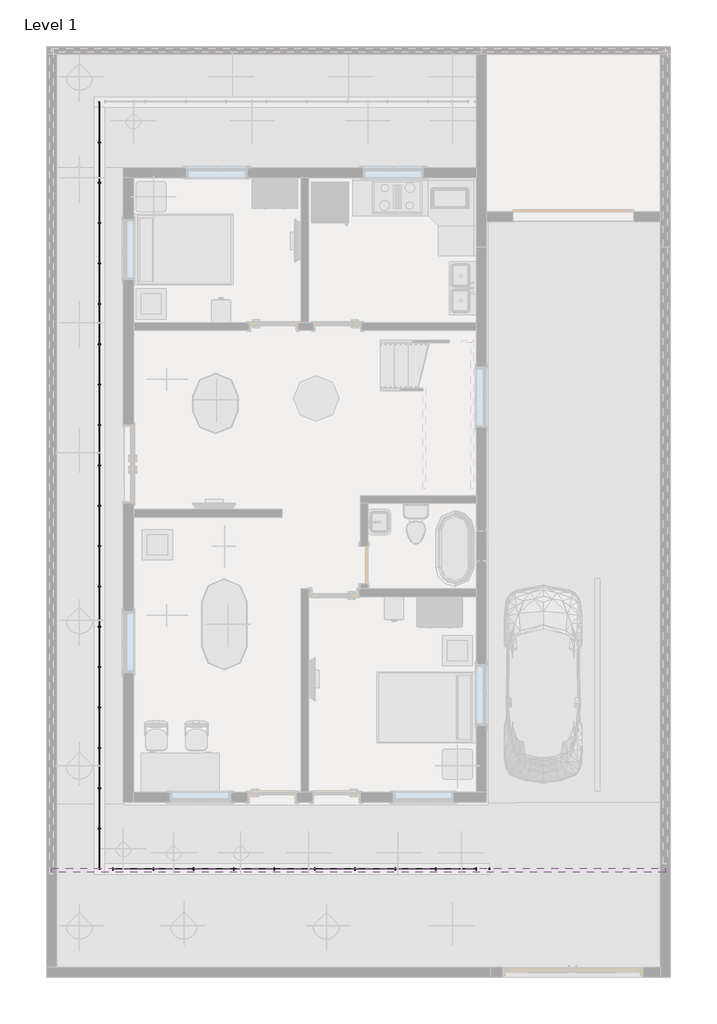
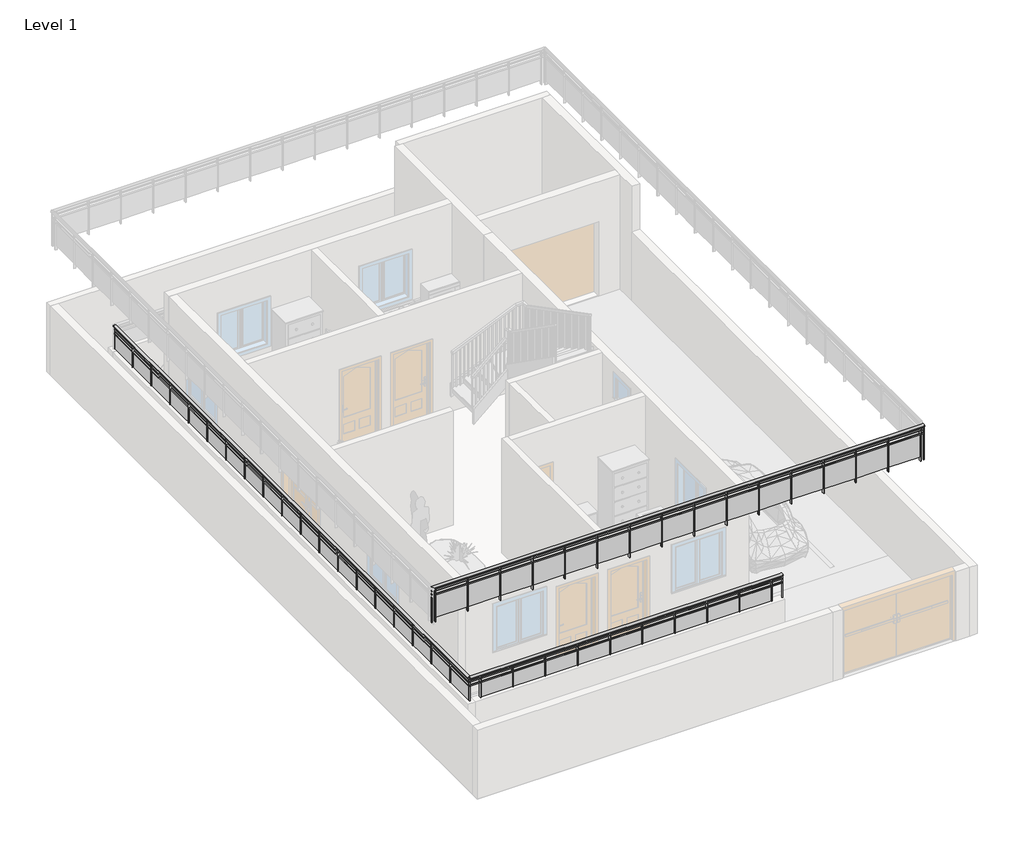
# One storey, part 2 of 5: 3 railings.
"""IFC4 building model written with IfcOpenShell, lengths in millimetres."""

from ifc_helpers import new_model, si_unit, point, frame, origin, place, context, project, spatial, polyline, ellipse_curve, trimmed, outline, extrude, element, save
from ifc_brep_helpers import plane_surface, extruded_surface, advanced_brep

model = new_model("IFC4")

# Units and contexts
model_context = context("Model", 3, world=origin())
ifc_project = project(units=[si_unit("LENGTHUNIT", "METRE", prefix="MILLI")], contexts=[model_context])

# Site, building, storey
site = spatial("IfcSite", under=ifc_project)
building = spatial("IfcBuilding", under=site)
storey = spatial("IfcBuildingStorey", under=building, Name="Level 1", Elevation=0.0)

# Railings
placement = place(None, origin())
element("IfcRailing", 1, ObjectType="Glass Panel - Bottom Fill", at=placement, inside=storey, context=model_context, shape_type="SolidModel", body=[
    advanced_brep(
    [(-10070.9350785, -4835.5966995, 1524.0), (-10070.9350785, -4911.7966995, 1524.0), (-2209.6350785, -4835.5966995, 1524.0), (-2209.6350785, -4911.7966995, 1524.0)],
    [
        (0, 1, ellipse_curve(frame((-10070.9350785, -4873.6966995, 1524.0), z_axis=(-1.0, 0.0, 0.0), x_axis=(0.0, -1.0, 0.0)), 38.1, 28.575)),
        (1, 0, ellipse_curve(frame((-10070.9350785, -4873.6966995, 1524.0), z_axis=(-1.0, 0.0, 0.0), x_axis=(0.0, -1.0, 0.0)), 38.1, 28.575)),
        (2, 3, ellipse_curve(frame((-2209.6350785, -4873.6966995, 1524.0), z_axis=(1.0, 0.0, 0.0), x_axis=(0.0, -1.0, 0.0)), 38.1, 28.575)),
        (3, 2, ellipse_curve(frame((-2209.6350785, -4873.6966995, 1524.0), z_axis=(1.0, 0.0, 0.0), x_axis=(0.0, -1.0, 0.0)), 38.1, 28.575)),
        (0, 2),
        (3, 1),
    ],
    [
        plane_surface(frame((-10070.9350785, -4873.6966995, 1524.0), z_axis=(-1.0, 0.0, 0.0), x_axis=(0.0, 1.0, 0.0))),
        plane_surface(frame((-2209.6350785, -4873.6966995, 1524.0), z_axis=(1.0, 0.0, 0.0), x_axis=(0.0, 1.0, 0.0))),
        extruded_surface(trimmed(ellipse_curve(frame((-2209.6350785, -4873.6966995, 1524.0), z_axis=(-1.0, 0.0, 0.0), x_axis=(0.0, -1.0, 0.0)), 38.1, 28.575), [point((-2209.6350785, -4835.5966995, 1524.0))], [point((-2209.6350785, -4911.7966995, 1524.0))], True, "CARTESIAN"), (-7861.300000000001, 0.0, 0.0), 7861.300000000001),
        extruded_surface(trimmed(ellipse_curve(frame((-2209.6350785, -4873.6966995, 1524.0), z_axis=(-1.0, 0.0, 0.0), x_axis=(0.0, -1.0, 0.0)), 38.1, 28.575), [point((-2209.6350785, -4911.7966995, 1524.0))], [point((-2209.6350785, -4835.5966995, 1524.0))], True, "CARTESIAN"), (-7861.300000000001, 0.0, 0.0), 7861.300000000001),
    ],
    [
        (0, [[1, 2]]),
        (1, [[3, 4]]),
        (2, [[-1, 5, -4, 6]]),
        (3, [[-2, -6, -3, -5]]),
    ],
),
    extrude(outline(polyline([(-10070.9350785, -4886.3966995), (-10070.9350785, -4860.9966995), (-2209.6350785, -4860.9966995), (-2209.6350785, -4886.3966995), (-10070.9350785, -4886.3966995)])), frame((0.0, 0.0, 1409.7), z_axis=(0.0, 0.0, 1.0), x_axis=(1.0, 0.0, 0.0)), (0.0, 0.0, 1.0), 25.4),
    extrude(outline(polyline([(-10070.9350785, -4886.3966995), (-10070.9350785, -4860.9966995), (-2209.6350785, -4860.9966995), (-2209.6350785, -4886.3966995), (-10070.9350785, -4886.3966995)])), frame((0.0, 0.0, 1308.1), z_axis=(0.0, 0.0, 1.0), x_axis=(1.0, 0.0, 0.0)), (0.0, 0.0, 1.0), 25.4),
    extrude(outline(polyline([(-2489.0350785, -4899.0966995), (-2489.0350785, -4848.2966995), (-2476.3350785, -4848.2966995), (-2476.3350785, -4899.0966995), (-2489.0350785, -4899.0966995)])), frame((0.0, 0.0, 609.6), z_axis=(0.0, 0.0, 1.0), x_axis=(1.0, 0.0, 0.0)), (0.0, 0.0, 1.0), 885.6788223),
    extrude(outline(polyline([(-3295.4850785, -4867.1615425), (-2482.6850785, -4867.1615425), (-2482.6850785, -4873.5115425), (-3295.4850785, -4873.5115425), (-3295.4850785, -4867.1615425)])), frame((0.0, 0.0, 711.2), z_axis=(0.0, 0.0, 1.0), x_axis=(1.0, 0.0, 0.0)), (0.0, 0.0, 1.0), 596.9),
    extrude(outline(polyline([(-3301.8350785, -4899.0966995), (-3301.8350785, -4848.2966995), (-3289.1350785, -4848.2966995), (-3289.1350785, -4899.0966995), (-3301.8350785, -4899.0966995)])), frame((0.0, 0.0, 609.6), z_axis=(0.0, 0.0, 1.0), x_axis=(1.0, 0.0, 0.0)), (0.0, 0.0, 1.0), 885.6788223),
    extrude(outline(polyline([(-4108.2850785, -4867.1615425), (-3295.4850785, -4867.1615425), (-3295.4850785, -4873.5115425), (-4108.2850785, -4873.5115425), (-4108.2850785, -4867.1615425)])), frame((0.0, 0.0, 711.2), z_axis=(0.0, 0.0, 1.0), x_axis=(1.0, 0.0, 0.0)), (0.0, 0.0, 1.0), 596.9),
    extrude(outline(polyline([(-4114.6350785, -4899.0966995), (-4114.6350785, -4848.2966995), (-4101.9350785, -4848.2966995), (-4101.9350785, -4899.0966995), (-4114.6350785, -4899.0966995)])), frame((0.0, 0.0, 609.6), z_axis=(0.0, 0.0, 1.0), x_axis=(1.0, 0.0, 0.0)), (0.0, 0.0, 1.0), 885.6788223),
    extrude(outline(polyline([(-4921.0850785, -4867.1615425), (-4108.2850785, -4867.1615425), (-4108.2850785, -4873.5115425), (-4921.0850785, -4873.5115425), (-4921.0850785, -4867.1615425)])), frame((0.0, 0.0, 711.2), z_axis=(0.0, 0.0, 1.0), x_axis=(1.0, 0.0, 0.0)), (0.0, 0.0, 1.0), 596.9),
    extrude(outline(polyline([(-4927.4350785, -4899.0966995), (-4927.4350785, -4848.2966995), (-4914.7350785, -4848.2966995), (-4914.7350785, -4899.0966995), (-4927.4350785, -4899.0966995)])), frame((0.0, 0.0, 609.6), z_axis=(0.0, 0.0, 1.0), x_axis=(1.0, 0.0, 0.0)), (0.0, 0.0, 1.0), 885.6788223),
    extrude(outline(polyline([(-5733.8850785, -4867.1615425), (-4921.0850785, -4867.1615425), (-4921.0850785, -4873.5115425), (-5733.8850785, -4873.5115425), (-5733.8850785, -4867.1615425)])), frame((0.0, 0.0, 711.2), z_axis=(0.0, 0.0, 1.0), x_axis=(1.0, 0.0, 0.0)), (0.0, 0.0, 1.0), 596.9),
    extrude(outline(polyline([(-5740.2350785, -4899.0966995), (-5740.2350785, -4848.2966995), (-5727.5350785, -4848.2966995), (-5727.5350785, -4899.0966995), (-5740.2350785, -4899.0966995)])), frame((0.0, 0.0, 609.6), z_axis=(0.0, 0.0, 1.0), x_axis=(1.0, 0.0, 0.0)), (0.0, 0.0, 1.0), 885.6788223),
    extrude(outline(polyline([(-6546.6850785, -4867.1615425), (-5733.8850785, -4867.1615425), (-5733.8850785, -4873.5115425), (-6546.6850785, -4873.5115425), (-6546.6850785, -4867.1615425)])), frame((0.0, 0.0, 711.2), z_axis=(0.0, 0.0, 1.0), x_axis=(1.0, 0.0, 0.0)), (0.0, 0.0, 1.0), 596.9),
    extrude(outline(polyline([(-6553.0350785, -4899.0966995), (-6553.0350785, -4848.2966995), (-6540.3350785, -4848.2966995), (-6540.3350785, -4899.0966995), (-6553.0350785, -4899.0966995)])), frame((0.0, 0.0, 609.6), z_axis=(0.0, 0.0, 1.0), x_axis=(1.0, 0.0, 0.0)), (0.0, 0.0, 1.0), 885.6788223),
    extrude(outline(polyline([(-7359.4850785, -4867.1615425), (-6546.6850785, -4867.1615425), (-6546.6850785, -4873.5115425), (-7359.4850785, -4873.5115425), (-7359.4850785, -4867.1615425)])), frame((0.0, 0.0, 711.2), z_axis=(0.0, 0.0, 1.0), x_axis=(1.0, 0.0, 0.0)), (0.0, 0.0, 1.0), 596.9),
    extrude(outline(polyline([(-7365.8350785, -4899.0966995), (-7365.8350785, -4848.2966995), (-7353.1350785, -4848.2966995), (-7353.1350785, -4899.0966995), (-7365.8350785, -4899.0966995)])), frame((0.0, 0.0, 609.6), z_axis=(0.0, 0.0, 1.0), x_axis=(1.0, 0.0, 0.0)), (0.0, 0.0, 1.0), 885.6788223),
    extrude(outline(polyline([(-8172.2850785, -4867.1615425), (-7359.4850785, -4867.1615425), (-7359.4850785, -4873.5115425), (-8172.2850785, -4873.5115425), (-8172.2850785, -4867.1615425)])), frame((0.0, 0.0, 711.2), z_axis=(0.0, 0.0, 1.0), x_axis=(1.0, 0.0, 0.0)), (0.0, 0.0, 1.0), 596.9),
    extrude(outline(polyline([(-8178.6350785, -4899.0966995), (-8178.6350785, -4848.2966995), (-8165.9350785, -4848.2966995), (-8165.9350785, -4899.0966995), (-8178.6350785, -4899.0966995)])), frame((0.0, 0.0, 609.6), z_axis=(0.0, 0.0, 1.0), x_axis=(1.0, 0.0, 0.0)), (0.0, 0.0, 1.0), 885.6788223),
    extrude(outline(polyline([(-8985.0850785, -4867.1615425), (-8172.2850785, -4867.1615425), (-8172.2850785, -4873.5115425), (-8985.0850785, -4873.5115425), (-8985.0850785, -4867.1615425)])), frame((0.0, 0.0, 711.2), z_axis=(0.0, 0.0, 1.0), x_axis=(1.0, 0.0, 0.0)), (0.0, 0.0, 1.0), 596.9),
    extrude(outline(polyline([(-8991.4350785, -4899.0966995), (-8991.4350785, -4848.2966995), (-8978.7350785, -4848.2966995), (-8978.7350785, -4899.0966995), (-8991.4350785, -4899.0966995)])), frame((0.0, 0.0, 609.6), z_axis=(0.0, 0.0, 1.0), x_axis=(1.0, 0.0, 0.0)), (0.0, 0.0, 1.0), 885.6788223),
    extrude(outline(polyline([(-9797.8850785, -4867.1615425), (-8985.0850785, -4867.1615425), (-8985.0850785, -4873.5115425), (-9797.8850785, -4873.5115425), (-9797.8850785, -4867.1615425)])), frame((0.0, 0.0, 711.2), z_axis=(0.0, 0.0, 1.0), x_axis=(1.0, 0.0, 0.0)), (0.0, 0.0, 1.0), 596.9),
    extrude(outline(polyline([(-9804.2350785, -4899.0966995), (-9804.2350785, -4848.2966995), (-9791.5350785, -4848.2966995), (-9791.5350785, -4899.0966995), (-9804.2350785, -4899.0966995)])), frame((0.0, 0.0, 609.6), z_axis=(0.0, 0.0, 1.0), x_axis=(1.0, 0.0, 0.0)), (0.0, 0.0, 1.0), 885.6788223),
    extrude(outline(polyline([(-2222.3350785, -4883.2216995), (-2222.3350785, -4864.1716995), (-2203.2850785, -4864.1716995), (-2203.2850785, -4883.2216995), (-2222.3350785, -4883.2216995)])), frame((0.0, 0.0, 609.6), z_axis=(0.0, 0.0, 1.0), x_axis=(1.0, 0.0, 0.0)), (0.0, 0.0, 1.0), 885.6788223),
    extrude(outline(polyline([(-10077.2850785, -4883.2216995), (-10077.2850785, -4864.1716995), (-10058.2350785, -4864.1716995), (-10058.2350785, -4883.2216995), (-10077.2850785, -4883.2216995)])), frame((0.0, 0.0, 609.6), z_axis=(0.0, 0.0, 1.0), x_axis=(1.0, 0.0, 0.0)), (0.0, 0.0, 1.0), 885.6788223),
])
element("IfcRailing", 2, ObjectType="Glass Panel - Bottom Fill", at=placement, inside=storey, context=model_context, shape_type="SolidModel", body=[
    advanced_brep(
    [(-10109.0350785, -4873.6966995, 1524.0), (-10032.8350785, -4873.6966995, 1524.0), (-10109.0350785, 10569.5033005, 1524.0), (-10032.8350785, 10569.5033005, 1524.0)],
    [
        (0, 1, ellipse_curve(frame((-10070.9350785, -4873.6966995, 1524.0), z_axis=(0.0, -1.0, 0.0), x_axis=(1.0, 0.0, 0.0)), 38.1, 28.575)),
        (1, 0, ellipse_curve(frame((-10070.9350785, -4873.6966995, 1524.0), z_axis=(0.0, -1.0, 0.0), x_axis=(1.0, 0.0, 0.0)), 38.1, 28.575)),
        (2, 3, ellipse_curve(frame((-10070.9350785, 10569.5033005, 1524.0), z_axis=(0.0, 1.0, 0.0), x_axis=(1.0, 0.0, 0.0)), 38.1, 28.575)),
        (3, 2, ellipse_curve(frame((-10070.9350785, 10569.5033005, 1524.0), z_axis=(0.0, 1.0, 0.0), x_axis=(1.0, 0.0, 0.0)), 38.1, 28.575)),
        (0, 2),
        (3, 1),
    ],
    [
        plane_surface(frame((-10070.9350785, -4873.6966995, 1524.0), z_axis=(0.0, -1.0, 0.0), x_axis=(0.0, 0.0, 1.0))),
        plane_surface(frame((-10070.9350785, 10569.5033005, 1524.0), z_axis=(0.0, 1.0, 0.0), x_axis=(0.0, 0.0, 1.0))),
        extruded_surface(trimmed(ellipse_curve(frame((-10070.9350785, 10569.5033005, 1524.0), z_axis=(0.0, -1.0, 0.0), x_axis=(1.0, 0.0, 0.0)), 38.1, 28.575), [point((-10109.0350785, 10569.5033005, 1524.0))], [point((-10032.8350785, 10569.5033005, 1524.0))], True, "CARTESIAN"), (0.0, -15443.2, 0.0), 15443.2),
        extruded_surface(trimmed(ellipse_curve(frame((-10070.9350785, 10569.5033005, 1524.0), z_axis=(0.0, -1.0, 0.0), x_axis=(1.0, 0.0, 0.0)), 38.1, 28.575), [point((-10032.8350785, 10569.5033005, 1524.0))], [point((-10109.0350785, 10569.5033005, 1524.0))], True, "CARTESIAN"), (0.0, -15443.2, 0.0), 15443.2),
    ],
    [
        (0, [[1, 2]]),
        (1, [[3, 4]]),
        (2, [[-1, 5, -4, 6]]),
        (3, [[-2, -6, -3, -5]]),
    ],
),
    extrude(outline(polyline([(-10058.2350785, -4873.6966995), (-10083.6350785, -4873.6966995), (-10083.6350785, 10569.5033005), (-10058.2350785, 10569.5033005), (-10058.2350785, -4873.6966995)])), frame((0.0, 0.0, 1409.7), z_axis=(0.0, 0.0, 1.0), x_axis=(1.0, 0.0, 0.0)), (0.0, 0.0, 1.0), 25.4),
    extrude(outline(polyline([(-10058.2350785, -4873.6966995), (-10083.6350785, -4873.6966995), (-10083.6350785, 10569.5033005), (-10058.2350785, 10569.5033005), (-10058.2350785, -4873.6966995)])), frame((0.0, 0.0, 1308.1), z_axis=(0.0, 0.0, 1.0), x_axis=(1.0, 0.0, 0.0)), (0.0, 0.0, 1.0), 25.4),
    extrude(outline(polyline([(-10077.4702355, 9756.7033005), (-10077.4702355, 10569.5033005), (-10071.1202355, 10569.5033005), (-10071.1202355, 9756.7033005), (-10077.4702355, 9756.7033005)])), frame((0.0, 0.0, 711.2), z_axis=(0.0, 0.0, 1.0), x_axis=(1.0, 0.0, 0.0)), (0.0, 0.0, 1.0), 596.9),
    extrude(outline(polyline([(-10045.5350785, 9750.3533005), (-10096.3350785, 9750.3533005), (-10096.3350785, 9763.0533005), (-10045.5350785, 9763.0533005), (-10045.5350785, 9750.3533005)])), frame((0.0, 0.0, 609.6), z_axis=(0.0, 0.0, 1.0), x_axis=(1.0, 0.0, 0.0)), (0.0, 0.0, 1.0), 885.6788223),
    extrude(outline(polyline([(-10077.4702355, 8943.9033005), (-10077.4702355, 9756.7033005), (-10071.1202355, 9756.7033005), (-10071.1202355, 8943.9033005), (-10077.4702355, 8943.9033005)])), frame((0.0, 0.0, 711.2), z_axis=(0.0, 0.0, 1.0), x_axis=(1.0, 0.0, 0.0)), (0.0, 0.0, 1.0), 596.9),
    extrude(outline(polyline([(-10045.5350785, 8937.5533005), (-10096.3350785, 8937.5533005), (-10096.3350785, 8950.2533005), (-10045.5350785, 8950.2533005), (-10045.5350785, 8937.5533005)])), frame((0.0, 0.0, 609.6), z_axis=(0.0, 0.0, 1.0), x_axis=(1.0, 0.0, 0.0)), (0.0, 0.0, 1.0), 885.6788223),
    extrude(outline(polyline([(-10077.4702355, 8131.1033005), (-10077.4702355, 8943.9033005), (-10071.1202355, 8943.9033005), (-10071.1202355, 8131.1033005), (-10077.4702355, 8131.1033005)])), frame((0.0, 0.0, 711.2), z_axis=(0.0, 0.0, 1.0), x_axis=(1.0, 0.0, 0.0)), (0.0, 0.0, 1.0), 596.9),
    extrude(outline(polyline([(-10045.5350785, 8124.7533005), (-10096.3350785, 8124.7533005), (-10096.3350785, 8137.4533005), (-10045.5350785, 8137.4533005), (-10045.5350785, 8124.7533005)])), frame((0.0, 0.0, 609.6), z_axis=(0.0, 0.0, 1.0), x_axis=(1.0, 0.0, 0.0)), (0.0, 0.0, 1.0), 885.6788223),
    extrude(outline(polyline([(-10077.4702355, 7318.3033005), (-10077.4702355, 8131.1033005), (-10071.1202355, 8131.1033005), (-10071.1202355, 7318.3033005), (-10077.4702355, 7318.3033005)])), frame((0.0, 0.0, 711.2), z_axis=(0.0, 0.0, 1.0), x_axis=(1.0, 0.0, 0.0)), (0.0, 0.0, 1.0), 596.9),
    extrude(outline(polyline([(-10045.5350785, 7311.9533005), (-10096.3350785, 7311.9533005), (-10096.3350785, 7324.6533005), (-10045.5350785, 7324.6533005), (-10045.5350785, 7311.9533005)])), frame((0.0, 0.0, 609.6), z_axis=(0.0, 0.0, 1.0), x_axis=(1.0, 0.0, 0.0)), (0.0, 0.0, 1.0), 885.6788223),
    extrude(outline(polyline([(-10077.4702355, 6505.5033005), (-10077.4702355, 7318.3033005), (-10071.1202355, 7318.3033005), (-10071.1202355, 6505.5033005), (-10077.4702355, 6505.5033005)])), frame((0.0, 0.0, 711.2), z_axis=(0.0, 0.0, 1.0), x_axis=(1.0, 0.0, 0.0)), (0.0, 0.0, 1.0), 596.9),
    extrude(outline(polyline([(-10045.5350785, 6499.1533005), (-10096.3350785, 6499.1533005), (-10096.3350785, 6511.8533005), (-10045.5350785, 6511.8533005), (-10045.5350785, 6499.1533005)])), frame((0.0, 0.0, 609.6), z_axis=(0.0, 0.0, 1.0), x_axis=(1.0, 0.0, 0.0)), (0.0, 0.0, 1.0), 885.6788223),
    extrude(outline(polyline([(-10077.4702355, 5692.7033005), (-10077.4702355, 6505.5033005), (-10071.1202355, 6505.5033005), (-10071.1202355, 5692.7033005), (-10077.4702355, 5692.7033005)])), frame((0.0, 0.0, 711.2), z_axis=(0.0, 0.0, 1.0), x_axis=(1.0, 0.0, 0.0)), (0.0, 0.0, 1.0), 596.9),
    extrude(outline(polyline([(-10045.5350785, 5686.3533005), (-10096.3350785, 5686.3533005), (-10096.3350785, 5699.0533005), (-10045.5350785, 5699.0533005), (-10045.5350785, 5686.3533005)])), frame((0.0, 0.0, 609.6), z_axis=(0.0, 0.0, 1.0), x_axis=(1.0, 0.0, 0.0)), (0.0, 0.0, 1.0), 885.6788223),
    extrude(outline(polyline([(-10077.4702355, 4879.9033005), (-10077.4702355, 5692.7033005), (-10071.1202355, 5692.7033005), (-10071.1202355, 4879.9033005), (-10077.4702355, 4879.9033005)])), frame((0.0, 0.0, 711.2), z_axis=(0.0, 0.0, 1.0), x_axis=(1.0, 0.0, 0.0)), (0.0, 0.0, 1.0), 596.9),
    extrude(outline(polyline([(-10045.5350785, 4873.5533005), (-10096.3350785, 4873.5533005), (-10096.3350785, 4886.2533005), (-10045.5350785, 4886.2533005), (-10045.5350785, 4873.5533005)])), frame((0.0, 0.0, 609.6), z_axis=(0.0, 0.0, 1.0), x_axis=(1.0, 0.0, 0.0)), (0.0, 0.0, 1.0), 885.6788223),
    extrude(outline(polyline([(-10077.4702355, 4067.1033005), (-10077.4702355, 4879.9033005), (-10071.1202355, 4879.9033005), (-10071.1202355, 4067.1033005), (-10077.4702355, 4067.1033005)])), frame((0.0, 0.0, 711.2), z_axis=(0.0, 0.0, 1.0), x_axis=(1.0, 0.0, 0.0)), (0.0, 0.0, 1.0), 596.9),
    extrude(outline(polyline([(-10045.5350785, 4060.7533005), (-10096.3350785, 4060.7533005), (-10096.3350785, 4073.4533005), (-10045.5350785, 4073.4533005), (-10045.5350785, 4060.7533005)])), frame((0.0, 0.0, 609.6), z_axis=(0.0, 0.0, 1.0), x_axis=(1.0, 0.0, 0.0)), (0.0, 0.0, 1.0), 885.6788223),
    extrude(outline(polyline([(-10077.4702355, 3254.3033005), (-10077.4702355, 4067.1033005), (-10071.1202355, 4067.1033005), (-10071.1202355, 3254.3033005), (-10077.4702355, 3254.3033005)])), frame((0.0, 0.0, 711.2), z_axis=(0.0, 0.0, 1.0), x_axis=(1.0, 0.0, 0.0)), (0.0, 0.0, 1.0), 596.9),
    extrude(outline(polyline([(-10045.5350785, 3247.9533005), (-10096.3350785, 3247.9533005), (-10096.3350785, 3260.6533005), (-10045.5350785, 3260.6533005), (-10045.5350785, 3247.9533005)])), frame((0.0, 0.0, 609.6), z_axis=(0.0, 0.0, 1.0), x_axis=(1.0, 0.0, 0.0)), (0.0, 0.0, 1.0), 885.6788223),
    extrude(outline(polyline([(-10077.4702355, 2441.5033005), (-10077.4702355, 3254.3033005), (-10071.1202355, 3254.3033005), (-10071.1202355, 2441.5033005), (-10077.4702355, 2441.5033005)])), frame((0.0, 0.0, 711.2), z_axis=(0.0, 0.0, 1.0), x_axis=(1.0, 0.0, 0.0)), (0.0, 0.0, 1.0), 596.9),
    extrude(outline(polyline([(-10045.5350785, 2435.1533005), (-10096.3350785, 2435.1533005), (-10096.3350785, 2447.8533005), (-10045.5350785, 2447.8533005), (-10045.5350785, 2435.1533005)])), frame((0.0, 0.0, 609.6), z_axis=(0.0, 0.0, 1.0), x_axis=(1.0, 0.0, 0.0)), (0.0, 0.0, 1.0), 885.6788223),
    extrude(outline(polyline([(-10077.4702355, 1628.7033005), (-10077.4702355, 2441.5033005), (-10071.1202355, 2441.5033005), (-10071.1202355, 1628.7033005), (-10077.4702355, 1628.7033005)])), frame((0.0, 0.0, 711.2), z_axis=(0.0, 0.0, 1.0), x_axis=(1.0, 0.0, 0.0)), (0.0, 0.0, 1.0), 596.9),
    extrude(outline(polyline([(-10045.5350785, 1622.3533005), (-10096.3350785, 1622.3533005), (-10096.3350785, 1635.0533005), (-10045.5350785, 1635.0533005), (-10045.5350785, 1622.3533005)])), frame((0.0, 0.0, 609.6), z_axis=(0.0, 0.0, 1.0), x_axis=(1.0, 0.0, 0.0)), (0.0, 0.0, 1.0), 885.6788223),
    extrude(outline(polyline([(-10077.4702355, 815.9033005), (-10077.4702355, 1628.7033005), (-10071.1202355, 1628.7033005), (-10071.1202355, 815.9033005), (-10077.4702355, 815.9033005)])), frame((0.0, 0.0, 711.2), z_axis=(0.0, 0.0, 1.0), x_axis=(1.0, 0.0, 0.0)), (0.0, 0.0, 1.0), 596.9),
    extrude(outline(polyline([(-10045.5350785, 809.5533005), (-10096.3350785, 809.5533005), (-10096.3350785, 822.2533005), (-10045.5350785, 822.2533005), (-10045.5350785, 809.5533005)])), frame((0.0, 0.0, 609.6), z_axis=(0.0, 0.0, 1.0), x_axis=(1.0, 0.0, 0.0)), (0.0, 0.0, 1.0), 885.6788223),
    extrude(outline(polyline([(-10077.4702355, 3.1033005), (-10077.4702355, 815.9033005), (-10071.1202355, 815.9033005), (-10071.1202355, 3.1033005), (-10077.4702355, 3.1033005)])), frame((0.0, 0.0, 711.2), z_axis=(0.0, 0.0, 1.0), x_axis=(1.0, 0.0, 0.0)), (0.0, 0.0, 1.0), 596.9),
    extrude(outline(polyline([(-10045.5350785, -3.2466995), (-10096.3350785, -3.2466995), (-10096.3350785, 9.4533005), (-10045.5350785, 9.4533005), (-10045.5350785, -3.2466995)])), frame((0.0, 0.0, 609.6), z_axis=(0.0, 0.0, 1.0), x_axis=(1.0, 0.0, 0.0)), (0.0, 0.0, 1.0), 885.6788223),
    extrude(outline(polyline([(-10077.4702355, -809.6966995), (-10077.4702355, 3.1033005), (-10071.1202355, 3.1033005), (-10071.1202355, -809.6966995), (-10077.4702355, -809.6966995)])), frame((0.0, 0.0, 711.2), z_axis=(0.0, 0.0, 1.0), x_axis=(1.0, 0.0, 0.0)), (0.0, 0.0, 1.0), 596.9),
    extrude(outline(polyline([(-10045.5350785, -816.0466995), (-10096.3350785, -816.0466995), (-10096.3350785, -803.3466995), (-10045.5350785, -803.3466995), (-10045.5350785, -816.0466995)])), frame((0.0, 0.0, 609.6), z_axis=(0.0, 0.0, 1.0), x_axis=(1.0, 0.0, 0.0)), (0.0, 0.0, 1.0), 885.6788223),
    extrude(outline(polyline([(-10077.4702355, -1622.4966995), (-10077.4702355, -809.6966995), (-10071.1202355, -809.6966995), (-10071.1202355, -1622.4966995), (-10077.4702355, -1622.4966995)])), frame((0.0, 0.0, 711.2), z_axis=(0.0, 0.0, 1.0), x_axis=(1.0, 0.0, 0.0)), (0.0, 0.0, 1.0), 596.9),
    extrude(outline(polyline([(-10045.5350785, -1628.8466995), (-10096.3350785, -1628.8466995), (-10096.3350785, -1616.1466995), (-10045.5350785, -1616.1466995), (-10045.5350785, -1628.8466995)])), frame((0.0, 0.0, 609.6), z_axis=(0.0, 0.0, 1.0), x_axis=(1.0, 0.0, 0.0)), (0.0, 0.0, 1.0), 885.6788223),
    extrude(outline(polyline([(-10077.4702355, -2435.2966995), (-10077.4702355, -1622.4966995), (-10071.1202355, -1622.4966995), (-10071.1202355, -2435.2966995), (-10077.4702355, -2435.2966995)])), frame((0.0, 0.0, 711.2), z_axis=(0.0, 0.0, 1.0), x_axis=(1.0, 0.0, 0.0)), (0.0, 0.0, 1.0), 596.9),
    extrude(outline(polyline([(-10045.5350785, -2441.6466995), (-10096.3350785, -2441.6466995), (-10096.3350785, -2428.9466995), (-10045.5350785, -2428.9466995), (-10045.5350785, -2441.6466995)])), frame((0.0, 0.0, 609.6), z_axis=(0.0, 0.0, 1.0), x_axis=(1.0, 0.0, 0.0)), (0.0, 0.0, 1.0), 885.6788223),
    extrude(outline(polyline([(-10077.4702355, -3248.0966995), (-10077.4702355, -2435.2966995), (-10071.1202355, -2435.2966995), (-10071.1202355, -3248.0966995), (-10077.4702355, -3248.0966995)])), frame((0.0, 0.0, 711.2), z_axis=(0.0, 0.0, 1.0), x_axis=(1.0, 0.0, 0.0)), (0.0, 0.0, 1.0), 596.9),
    extrude(outline(polyline([(-10045.5350785, -3254.4466995), (-10096.3350785, -3254.4466995), (-10096.3350785, -3241.7466995), (-10045.5350785, -3241.7466995), (-10045.5350785, -3254.4466995)])), frame((0.0, 0.0, 609.6), z_axis=(0.0, 0.0, 1.0), x_axis=(1.0, 0.0, 0.0)), (0.0, 0.0, 1.0), 885.6788223),
    extrude(outline(polyline([(-10077.4702355, -4060.8966995), (-10077.4702355, -3248.0966995), (-10071.1202355, -3248.0966995), (-10071.1202355, -4060.8966995), (-10077.4702355, -4060.8966995)])), frame((0.0, 0.0, 711.2), z_axis=(0.0, 0.0, 1.0), x_axis=(1.0, 0.0, 0.0)), (0.0, 0.0, 1.0), 596.9),
    extrude(outline(polyline([(-10045.5350785, -4067.2466995), (-10096.3350785, -4067.2466995), (-10096.3350785, -4054.5466995), (-10045.5350785, -4054.5466995), (-10045.5350785, -4067.2466995)])), frame((0.0, 0.0, 609.6), z_axis=(0.0, 0.0, 1.0), x_axis=(1.0, 0.0, 0.0)), (0.0, 0.0, 1.0), 885.6788223),
    extrude(outline(polyline([(-10077.4702355, -4873.6966995), (-10077.4702355, -4060.8966995), (-10071.1202355, -4060.8966995), (-10071.1202355, -4873.6966995), (-10077.4702355, -4873.6966995)])), frame((0.0, 0.0, 711.2), z_axis=(0.0, 0.0, 1.0), x_axis=(1.0, 0.0, 0.0)), (0.0, 0.0, 1.0), 596.9),
    extrude(outline(polyline([(-10061.4100785, 10556.8033005), (-10080.4600785, 10556.8033005), (-10080.4600785, 10575.8533005), (-10061.4100785, 10575.8533005), (-10061.4100785, 10556.8033005)])), frame((0.0, 0.0, 609.6), z_axis=(0.0, 0.0, 1.0), x_axis=(1.0, 0.0, 0.0)), (0.0, 0.0, 1.0), 885.6788223),
    extrude(outline(polyline([(-10061.4100785, -4880.0466995), (-10080.4600785, -4880.0466995), (-10080.4600785, -4860.9966995), (-10061.4100785, -4860.9966995), (-10061.4100785, -4880.0466995)])), frame((0.0, 0.0, 609.6), z_axis=(0.0, 0.0, 1.0), x_axis=(1.0, 0.0, 0.0)), (0.0, 0.0, 1.0), 885.6788223),
])
element("IfcRailing", 3, ObjectType="Glass Panel - Bottom Fill", at=placement, inside=storey, context=model_context, shape_type="SolidModel", body=[
    advanced_brep(
    [(-11036.1350785, -4860.9966995, 4267.2), (-11036.1350785, -4937.1966995, 4267.2), (1333.6649215, -4860.9966995, 4267.2), (1333.6649215, -4937.1966995, 4267.2)],
    [
        (0, 1, ellipse_curve(frame((-11036.1350785, -4899.0966995, 4267.2), z_axis=(-1.0, 0.0, 0.0), x_axis=(0.0, -1.0, 0.0)), 38.1, 28.575)),
        (1, 0, ellipse_curve(frame((-11036.1350785, -4899.0966995, 4267.2), z_axis=(-1.0, 0.0, 0.0), x_axis=(0.0, -1.0, 0.0)), 38.1, 28.575)),
        (2, 3, ellipse_curve(frame((1333.6649215, -4899.0966995, 4267.2), z_axis=(1.0, 0.0, 0.0), x_axis=(0.0, -1.0, 0.0)), 38.1, 28.575)),
        (3, 2, ellipse_curve(frame((1333.6649215, -4899.0966995, 4267.2), z_axis=(1.0, 0.0, 0.0), x_axis=(0.0, -1.0, 0.0)), 38.1, 28.575)),
        (0, 2),
        (3, 1),
    ],
    [
        plane_surface(frame((-11036.1350785, -4899.0966995, 4267.2), z_axis=(-1.0, 0.0, 0.0), x_axis=(0.0, 1.0, 0.0))),
        plane_surface(frame((1333.6649215, -4899.0966995, 4267.2), z_axis=(1.0, 0.0, 0.0), x_axis=(0.0, 1.0, 0.0))),
        extruded_surface(trimmed(ellipse_curve(frame((1333.6649215, -4899.0966995, 4267.2), z_axis=(-1.0, 0.0, 0.0), x_axis=(0.0, -1.0, 0.0)), 38.1, 28.575), [point((1333.6649215, -4860.9966995, 4267.2))], [point((1333.6649215, -4937.1966995, 4267.2))], True, "CARTESIAN"), (-12369.8, 0.0, 0.0), 12369.8),
        extruded_surface(trimmed(ellipse_curve(frame((1333.6649215, -4899.0966995, 4267.2), z_axis=(-1.0, 0.0, 0.0), x_axis=(0.0, -1.0, 0.0)), 38.1, 28.575), [point((1333.6649215, -4937.1966995, 4267.2))], [point((1333.6649215, -4860.9966995, 4267.2))], True, "CARTESIAN"), (-12369.8, 0.0, 0.0), 12369.8),
    ],
    [
        (0, [[1, 2]]),
        (1, [[3, 4]]),
        (2, [[-1, 5, -4, 6]]),
        (3, [[-2, -6, -3, -5]]),
    ],
),
    extrude(outline(polyline([(-11036.1350785, -4911.7966995), (-11036.1350785, -4886.3966995), (1333.6649215, -4886.3966995), (1333.6649215, -4911.7966995), (-11036.1350785, -4911.7966995)])), frame((0.0, 0.0, 4152.9), z_axis=(0.0, 0.0, 1.0), x_axis=(1.0, 0.0, 0.0)), (0.0, 0.0, 1.0), 25.4),
    extrude(outline(polyline([(-11036.1350785, -4911.7966995), (-11036.1350785, -4886.3966995), (1333.6649215, -4886.3966995), (1333.6649215, -4911.7966995), (-11036.1350785, -4911.7966995)])), frame((0.0, 0.0, 4051.3), z_axis=(0.0, 0.0, 1.0), x_axis=(1.0, 0.0, 0.0)), (0.0, 0.0, 1.0), 25.4),
    extrude(outline(polyline([(1238.4149215, -4924.4966995), (1238.4149215, -4873.6966995), (1251.1149215, -4873.6966995), (1251.1149215, -4924.4966995), (1238.4149215, -4924.4966995)])), frame((0.0, 0.0, 3352.8), z_axis=(0.0, 0.0, 1.0), x_axis=(1.0, 0.0, 0.0)), (0.0, 0.0, 1.0), 885.6788223),
    extrude(outline(polyline([(431.9649215, -4892.5615425), (1244.7649215, -4892.5615425), (1244.7649215, -4898.9115425), (431.9649215, -4898.9115425), (431.9649215, -4892.5615425)])), frame((0.0, 0.0, 3454.4), z_axis=(0.0, 0.0, 1.0), x_axis=(1.0, 0.0, 0.0)), (0.0, 0.0, 1.0), 596.9),
    extrude(outline(polyline([(425.6149215, -4924.4966995), (425.6149215, -4873.6966995), (438.3149215, -4873.6966995), (438.3149215, -4924.4966995), (425.6149215, -4924.4966995)])), frame((0.0, 0.0, 3352.8), z_axis=(0.0, 0.0, 1.0), x_axis=(1.0, 0.0, 0.0)), (0.0, 0.0, 1.0), 885.6788223),
    extrude(outline(polyline([(-380.8350785, -4892.5615425), (431.9649215, -4892.5615425), (431.9649215, -4898.9115425), (-380.8350785, -4898.9115425), (-380.8350785, -4892.5615425)])), frame((0.0, 0.0, 3454.4), z_axis=(0.0, 0.0, 1.0), x_axis=(1.0, 0.0, 0.0)), (0.0, 0.0, 1.0), 596.9),
    extrude(outline(polyline([(-387.1850785, -4924.4966995), (-387.1850785, -4873.6966995), (-374.4850785, -4873.6966995), (-374.4850785, -4924.4966995), (-387.1850785, -4924.4966995)])), frame((0.0, 0.0, 3352.8), z_axis=(0.0, 0.0, 1.0), x_axis=(1.0, 0.0, 0.0)), (0.0, 0.0, 1.0), 885.6788223),
    extrude(outline(polyline([(-1193.6350785, -4892.5615425), (-380.8350785, -4892.5615425), (-380.8350785, -4898.9115425), (-1193.6350785, -4898.9115425), (-1193.6350785, -4892.5615425)])), frame((0.0, 0.0, 3454.4), z_axis=(0.0, 0.0, 1.0), x_axis=(1.0, 0.0, 0.0)), (0.0, 0.0, 1.0), 596.9),
    extrude(outline(polyline([(-1199.9850785, -4924.4966995), (-1199.9850785, -4873.6966995), (-1187.2850785, -4873.6966995), (-1187.2850785, -4924.4966995), (-1199.9850785, -4924.4966995)])), frame((0.0, 0.0, 3352.8), z_axis=(0.0, 0.0, 1.0), x_axis=(1.0, 0.0, 0.0)), (0.0, 0.0, 1.0), 885.6788223),
    extrude(outline(polyline([(-2006.4350785, -4892.5615425), (-1193.6350785, -4892.5615425), (-1193.6350785, -4898.9115425), (-2006.4350785, -4898.9115425), (-2006.4350785, -4892.5615425)])), frame((0.0, 0.0, 3454.4), z_axis=(0.0, 0.0, 1.0), x_axis=(1.0, 0.0, 0.0)), (0.0, 0.0, 1.0), 596.9),
    extrude(outline(polyline([(-2012.7850785, -4924.4966995), (-2012.7850785, -4873.6966995), (-2000.0850785, -4873.6966995), (-2000.0850785, -4924.4966995), (-2012.7850785, -4924.4966995)])), frame((0.0, 0.0, 3352.8), z_axis=(0.0, 0.0, 1.0), x_axis=(1.0, 0.0, 0.0)), (0.0, 0.0, 1.0), 885.6788223),
    extrude(outline(polyline([(-2819.2350785, -4892.5615425), (-2006.4350785, -4892.5615425), (-2006.4350785, -4898.9115425), (-2819.2350785, -4898.9115425), (-2819.2350785, -4892.5615425)])), frame((0.0, 0.0, 3454.4), z_axis=(0.0, 0.0, 1.0), x_axis=(1.0, 0.0, 0.0)), (0.0, 0.0, 1.0), 596.9),
    extrude(outline(polyline([(-2825.5850785, -4924.4966995), (-2825.5850785, -4873.6966995), (-2812.8850785, -4873.6966995), (-2812.8850785, -4924.4966995), (-2825.5850785, -4924.4966995)])), frame((0.0, 0.0, 3352.8), z_axis=(0.0, 0.0, 1.0), x_axis=(1.0, 0.0, 0.0)), (0.0, 0.0, 1.0), 885.6788223),
    extrude(outline(polyline([(-3632.0350785, -4892.5615425), (-2819.2350785, -4892.5615425), (-2819.2350785, -4898.9115425), (-3632.0350785, -4898.9115425), (-3632.0350785, -4892.5615425)])), frame((0.0, 0.0, 3454.4), z_axis=(0.0, 0.0, 1.0), x_axis=(1.0, 0.0, 0.0)), (0.0, 0.0, 1.0), 596.9),
    extrude(outline(polyline([(-3638.3850785, -4924.4966995), (-3638.3850785, -4873.6966995), (-3625.6850785, -4873.6966995), (-3625.6850785, -4924.4966995), (-3638.3850785, -4924.4966995)])), frame((0.0, 0.0, 3352.8), z_axis=(0.0, 0.0, 1.0), x_axis=(1.0, 0.0, 0.0)), (0.0, 0.0, 1.0), 885.6788223),
    extrude(outline(polyline([(-4444.8350785, -4892.5615425), (-3632.0350785, -4892.5615425), (-3632.0350785, -4898.9115425), (-4444.8350785, -4898.9115425), (-4444.8350785, -4892.5615425)])), frame((0.0, 0.0, 3454.4), z_axis=(0.0, 0.0, 1.0), x_axis=(1.0, 0.0, 0.0)), (0.0, 0.0, 1.0), 596.9),
    extrude(outline(polyline([(-4451.1850785, -4924.4966995), (-4451.1850785, -4873.6966995), (-4438.4850785, -4873.6966995), (-4438.4850785, -4924.4966995), (-4451.1850785, -4924.4966995)])), frame((0.0, 0.0, 3352.8), z_axis=(0.0, 0.0, 1.0), x_axis=(1.0, 0.0, 0.0)), (0.0, 0.0, 1.0), 885.6788223),
    extrude(outline(polyline([(-5257.6350785, -4892.5615425), (-4444.8350785, -4892.5615425), (-4444.8350785, -4898.9115425), (-5257.6350785, -4898.9115425), (-5257.6350785, -4892.5615425)])), frame((0.0, 0.0, 3454.4), z_axis=(0.0, 0.0, 1.0), x_axis=(1.0, 0.0, 0.0)), (0.0, 0.0, 1.0), 596.9),
    extrude(outline(polyline([(-5263.9850785, -4924.4966995), (-5263.9850785, -4873.6966995), (-5251.2850785, -4873.6966995), (-5251.2850785, -4924.4966995), (-5263.9850785, -4924.4966995)])), frame((0.0, 0.0, 3352.8), z_axis=(0.0, 0.0, 1.0), x_axis=(1.0, 0.0, 0.0)), (0.0, 0.0, 1.0), 885.6788223),
    extrude(outline(polyline([(-6070.4350785, -4892.5615425), (-5257.6350785, -4892.5615425), (-5257.6350785, -4898.9115425), (-6070.4350785, -4898.9115425), (-6070.4350785, -4892.5615425)])), frame((0.0, 0.0, 3454.4), z_axis=(0.0, 0.0, 1.0), x_axis=(1.0, 0.0, 0.0)), (0.0, 0.0, 1.0), 596.9),
    extrude(outline(polyline([(-6076.7850785, -4924.4966995), (-6076.7850785, -4873.6966995), (-6064.0850785, -4873.6966995), (-6064.0850785, -4924.4966995), (-6076.7850785, -4924.4966995)])), frame((0.0, 0.0, 3352.8), z_axis=(0.0, 0.0, 1.0), x_axis=(1.0, 0.0, 0.0)), (0.0, 0.0, 1.0), 885.6788223),
    extrude(outline(polyline([(-6883.2350785, -4892.5615425), (-6070.4350785, -4892.5615425), (-6070.4350785, -4898.9115425), (-6883.2350785, -4898.9115425), (-6883.2350785, -4892.5615425)])), frame((0.0, 0.0, 3454.4), z_axis=(0.0, 0.0, 1.0), x_axis=(1.0, 0.0, 0.0)), (0.0, 0.0, 1.0), 596.9),
    extrude(outline(polyline([(-6889.5850785, -4924.4966995), (-6889.5850785, -4873.6966995), (-6876.8850785, -4873.6966995), (-6876.8850785, -4924.4966995), (-6889.5850785, -4924.4966995)])), frame((0.0, 0.0, 3352.8), z_axis=(0.0, 0.0, 1.0), x_axis=(1.0, 0.0, 0.0)), (0.0, 0.0, 1.0), 885.6788223),
    extrude(outline(polyline([(-7696.0350785, -4892.5615425), (-6883.2350785, -4892.5615425), (-6883.2350785, -4898.9115425), (-7696.0350785, -4898.9115425), (-7696.0350785, -4892.5615425)])), frame((0.0, 0.0, 3454.4), z_axis=(0.0, 0.0, 1.0), x_axis=(1.0, 0.0, 0.0)), (0.0, 0.0, 1.0), 596.9),
    extrude(outline(polyline([(-7702.3850785, -4924.4966995), (-7702.3850785, -4873.6966995), (-7689.6850785, -4873.6966995), (-7689.6850785, -4924.4966995), (-7702.3850785, -4924.4966995)])), frame((0.0, 0.0, 3352.8), z_axis=(0.0, 0.0, 1.0), x_axis=(1.0, 0.0, 0.0)), (0.0, 0.0, 1.0), 885.6788223),
    extrude(outline(polyline([(-8508.8350785, -4892.5615425), (-7696.0350785, -4892.5615425), (-7696.0350785, -4898.9115425), (-8508.8350785, -4898.9115425), (-8508.8350785, -4892.5615425)])), frame((0.0, 0.0, 3454.4), z_axis=(0.0, 0.0, 1.0), x_axis=(1.0, 0.0, 0.0)), (0.0, 0.0, 1.0), 596.9),
    extrude(outline(polyline([(-8515.1850785, -4924.4966995), (-8515.1850785, -4873.6966995), (-8502.4850785, -4873.6966995), (-8502.4850785, -4924.4966995), (-8515.1850785, -4924.4966995)])), frame((0.0, 0.0, 3352.8), z_axis=(0.0, 0.0, 1.0), x_axis=(1.0, 0.0, 0.0)), (0.0, 0.0, 1.0), 885.6788223),
    extrude(outline(polyline([(-9321.6350785, -4892.5615425), (-8508.8350785, -4892.5615425), (-8508.8350785, -4898.9115425), (-9321.6350785, -4898.9115425), (-9321.6350785, -4892.5615425)])), frame((0.0, 0.0, 3454.4), z_axis=(0.0, 0.0, 1.0), x_axis=(1.0, 0.0, 0.0)), (0.0, 0.0, 1.0), 596.9),
    extrude(outline(polyline([(-9327.9850785, -4924.4966995), (-9327.9850785, -4873.6966995), (-9315.2850785, -4873.6966995), (-9315.2850785, -4924.4966995), (-9327.9850785, -4924.4966995)])), frame((0.0, 0.0, 3352.8), z_axis=(0.0, 0.0, 1.0), x_axis=(1.0, 0.0, 0.0)), (0.0, 0.0, 1.0), 885.6788223),
    extrude(outline(polyline([(-10134.4350785, -4892.5615425), (-9321.6350785, -4892.5615425), (-9321.6350785, -4898.9115425), (-10134.4350785, -4898.9115425), (-10134.4350785, -4892.5615425)])), frame((0.0, 0.0, 3454.4), z_axis=(0.0, 0.0, 1.0), x_axis=(1.0, 0.0, 0.0)), (0.0, 0.0, 1.0), 596.9),
    extrude(outline(polyline([(-10140.7850785, -4924.4966995), (-10140.7850785, -4873.6966995), (-10128.0850785, -4873.6966995), (-10128.0850785, -4924.4966995), (-10140.7850785, -4924.4966995)])), frame((0.0, 0.0, 3352.8), z_axis=(0.0, 0.0, 1.0), x_axis=(1.0, 0.0, 0.0)), (0.0, 0.0, 1.0), 885.6788223),
    extrude(outline(polyline([(-10947.2350785, -4892.5615425), (-10134.4350785, -4892.5615425), (-10134.4350785, -4898.9115425), (-10947.2350785, -4898.9115425), (-10947.2350785, -4892.5615425)])), frame((0.0, 0.0, 3454.4), z_axis=(0.0, 0.0, 1.0), x_axis=(1.0, 0.0, 0.0)), (0.0, 0.0, 1.0), 596.9),
    extrude(outline(polyline([(-10953.5850785, -4924.4966995), (-10953.5850785, -4873.6966995), (-10940.8850785, -4873.6966995), (-10940.8850785, -4924.4966995), (-10953.5850785, -4924.4966995)])), frame((0.0, 0.0, 3352.8), z_axis=(0.0, 0.0, 1.0), x_axis=(1.0, 0.0, 0.0)), (0.0, 0.0, 1.0), 885.6788223),
    extrude(outline(polyline([(1320.9649215, -4908.6216995), (1320.9649215, -4889.5716995), (1340.0149215, -4889.5716995), (1340.0149215, -4908.6216995), (1320.9649215, -4908.6216995)])), frame((0.0, 0.0, 3352.8), z_axis=(0.0, 0.0, 1.0), x_axis=(1.0, 0.0, 0.0)), (0.0, 0.0, 1.0), 885.6788223),
    extrude(outline(polyline([(-11042.4850785, -4908.6216995), (-11042.4850785, -4889.5716995), (-11023.4350785, -4889.5716995), (-11023.4350785, -4908.6216995), (-11042.4850785, -4908.6216995)])), frame((0.0, 0.0, 3352.8), z_axis=(0.0, 0.0, 1.0), x_axis=(1.0, 0.0, 0.0)), (0.0, 0.0, 1.0), 885.6788223),
])

save(model, "model.ifc")

# Revit data of these elements
# Type "Glass Panel - Bottom Fill"
#   Assembly Code = "C2010400"
#   built-in parameter 1008612 = 0.0416667 (stored number, unit not read)
#   built-in parameter 1008611 = 0.0416667 (stored number, unit not read)
#   built-in parameter 1008609 = 0.333333 (stored number, unit not read)
#   built-in parameter 1008604 = 0.166667 (stored number, unit not read)
#   built-in parameter 1008603 = 0.166667 (stored number, unit not read)
#   Railing Height = 3' - 0"
#   built-in parameter 1008630 = 2
#   built-in parameter 1008610 = 2
#   built-in parameter 1008618 = Baluster - Square : 3/4"
# Elements 1, 2 (IfcRailing, "Glass Panel - Bottom Fill")
#   built-in parameter 1008621 = 2 (stored number, unit not read)
#   Phase Created = New Construction
#   Materials on its faces: "Glass"
# Element 3 (IfcRailing, "Glass Panel - Bottom Fill")
#   built-in parameter 1008621 = 11 (stored number, unit not read)
#   Phase Created = New Construction
#   Materials on its faces: "Glass"
# Materials
#   "Glass": class "Glass", colour RGB 0 128 192, transparency 0.75, Description = "Soda Lime Glass", Cost = 0
